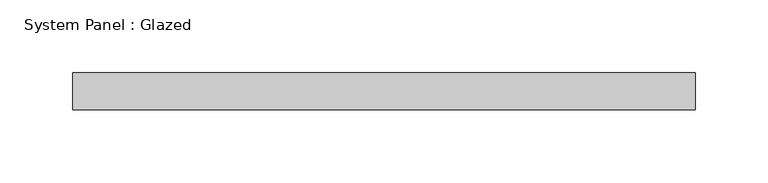
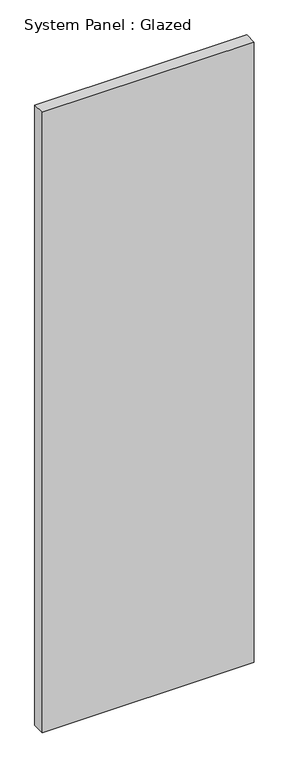
"""IFC4 building model written with IfcOpenShell, lengths in millimetres: plate geometry, System Panel : Glazed."""

from ifc_helpers import new_model, si_unit, origin, origin_with_axes, place, context, project, spatial, polyline, outline, extrude, source, transform, mapped, element, save


def system_panel_glazed_cae65973(model_context):
    return source(origin(), model_context, "Body", "SweptSolid", [
        extrude(outline(polyline([(214.3125, 19.05), (-214.3125, 19.05), (-214.3125, 44.45), (214.3125, 44.45), (214.3125, 19.05)])), origin_with_axes(), (0.0, 0.0, 1.0), 1325.5193485),
    ])


if __name__ == "__main__":
    model = new_model("IFC4")
    model_context = context("Model", 3, world=origin())
    ifc_project = project(units=[si_unit("LENGTHUNIT", "METRE", prefix="MILLI")], contexts=[model_context])
    site = spatial("IfcSite", under=ifc_project)
    building = spatial("IfcBuilding", under=site)
    placement = place(None, origin())
    system_panel_glazed_shape = system_panel_glazed_cae65973(model_context)
    element("IfcPlate", 1, ObjectType="System Panel : Glazed", at=placement, inside=building, context=model_context, shape_type="MappedRepresentation", body=[
        mapped(system_panel_glazed_shape, transform((0.0, 0.0, 0.0), x_axis=(1.0, 0.0, 0.0), y_axis=(0.0, 1.0, 0.0), z_axis=(0.0, 0.0, 1.0))),
    ])
    save(model, "model.ifc")

# Revit data of these elements
# Type "System Panel : Glazed"
#   Construction Type Id = "GSP4R"
#   Analytic Construction = "1/8 in Pilkington single glazing"
#   Visual Light Transmittance = 0.9
#   Solar Heat Gain Coefficient = 0.86
#   Heat Transfer Coefficient (U) = 1.18115 BTU/(h·ft²·°F)
#   Define Thermal Properties by = 1
# Element 1 (IfcPlate, "System Panel : Glazed")
#   Materials on its faces: "Glass"
# Materials
#   "Glass": class "Glass", colour RGB 0 128 192, transparency 0.75, Description = "Soda Lime Glass", Cost = 0
